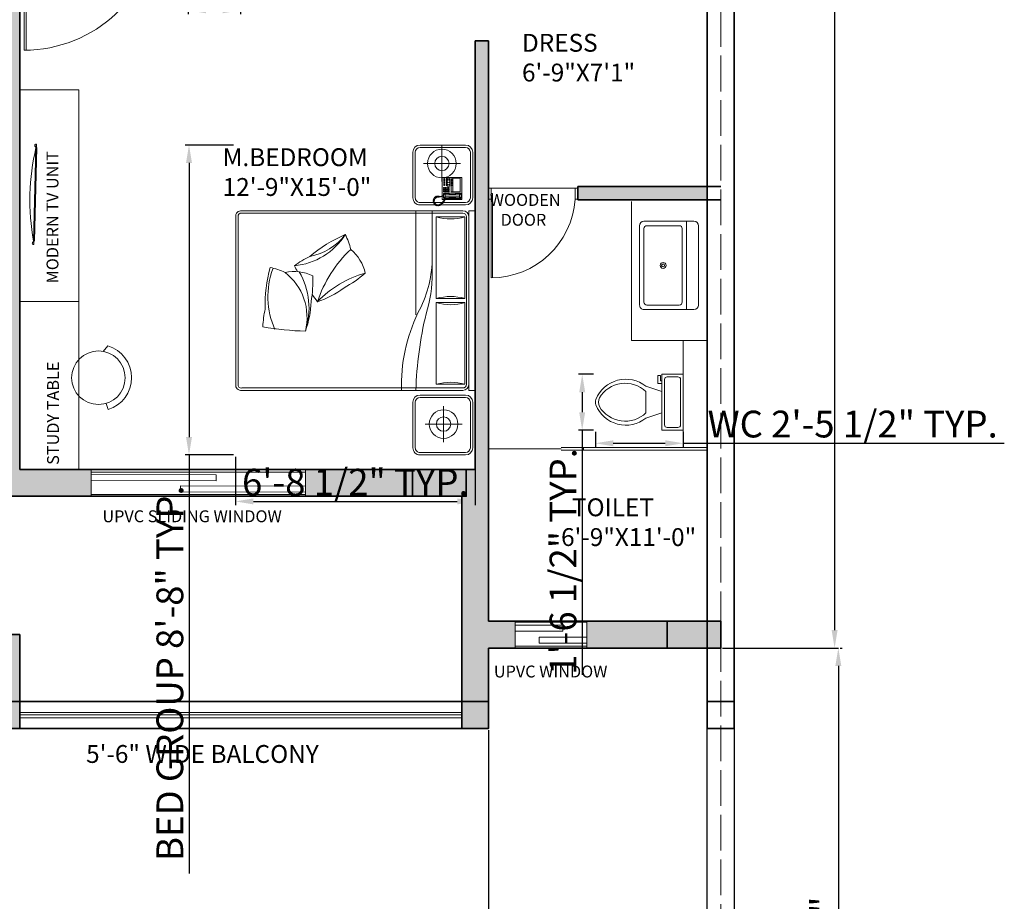
# Model space of a CAD drawing. Units: millimetres. Extents: x 595116 to 630915, y 909473 to 920225.
# Tile 131 of 134: x 630585 to 630915, y 919276 to 919572. Entities that reach past the tile are written whole.
import ezdxf

# ---------------------------------------------------------------- set-up
doc = ezdxf.new("R2010")
doc.units = ezdxf.units.MM
doc.linetypes.add('ACAD_ISO02W100', pattern=[15, 12, -3])
for name, color, linetype, lineweight in [('A-AREA-IDEN', 7, 'Continuous', 20), ('A-EQPM', 8, 'Continuous', 13), ('A-FLOR-BALC', 152, 'Continuous', 18), ('A-FLOR-FIXT', 9, 'Continuous', 18), ('A-FURN', 32, 'Continuous', 18), ('A-WALL', 1, 'Continuous', 35), ('A-WALL-PATT', 8, 'Continuous', 13), ('C-PROP', 7, 'Continuous', 25), ('C-PROP-REF', 240, 'ACAD_ISO02W100', 13), ('Column', 6, 'Continuous', 35), ('Dimension', 3, 'Continuous', 18), ('Doors', 31, 'Continuous', 20), ('Text', 7, 'Continuous', 18), ('Windows', 33, 'Continuous', 18)]:
    doc.layers.add(name, color=color, linetype=linetype, lineweight=lineweight)
doc.styles.get("Standard").update_dxf_attribs({"font": 'arial.ttf'})
doc.dimstyles.new('ISO-25', dxfattribs={"dimtxt": 9, "dimasz": 6, "dimexe": 1.25, "dimexo": 0.625, "dimtad": 1, "dimlunit": 4, "dimtxsty": 'Standard', "dimcen": 2.5, "dimadec": 0, "dimazin": 0, "dimtfac": 1, "dimtmove": 0, "dimatfit": 3, "dimfxl": 1, "dimarcsym": 0})

# ---------------------------------------------------------------- blocks, each defined once
blk = doc.blocks.new('KWD')
for points in [[(629753.63, 919957.93), (629752.54, 919957.93), (629752.54, 919953.43), (629753.63, 919953.43)], [(629787.45, 919957.93), (629787.45, 919953.43), (629788.54, 919953.43), (629788.54, 919957.93)]]:
    blk.add_lwpolyline(points, close=True)
blk.add_lwpolyline([(629753.63, 919921.79), (629753.63, 919955.68), (629754.13, 919955.68), (629754.13, 919921.8)])
blk.add_arc((629753.64, 919955.68), 33.88, 269.99, 356.196)
blk = doc.blocks.new('DS')
blk.add_lwpolyline([(630069.78, 919993.92), (630069.78, 919965.68), (630069.37, 919965.68), (630069.37, 919993.91)])
for points in [[(630041.6, 919963.81), (630041.6, 919967.56), (630040.69, 919967.56), (630040.69, 919963.81)], [(630069.78, 919963.81), (630070.69, 919963.81), (630070.69, 919967.56), (630069.78, 919967.56)]]:
    blk.add_lwpolyline(points, close=True)
blk.add_arc((630069.78, 919965.69), 28.24, 89.99, 176.196)
blk = doc.blocks.new('Toilet - top')
for p, q in [((9.5, -6), (9.5, -2)), ((-10, -8.5), (-8, -8.5)), ((-10, -9.5), (-10, -8.5)), ((-7, -9.5), (-10, -9.5)), ((-8, -8.5), (-8, -8)), ((-7, -8), (-7, -9.5)), ((-4, -8), (-6, -14)), ((4, -8), (6, -14)), ((4, -14), (-4, -14))]:
    blk.add_line(p, q)
blk.add_lwpolyline([(10.5, -8), (10.5, 0), (-10.5, 0), (-10.5, -8)], close=True)
for points in [[(-9.5, -2), (-9.5, -6)], [(8.5, -1), (-8.5, -1)], [(-8.5, -7), (8.5, -7)]]:
    blk.add_lwpolyline(points)
for centre, radius, start, end in [((-8.62, -1.88), 0.884, 81.8699, 188.1301), ((8.62, -1.88), 0.884, 351.8699, 98.1301), ((-8.62, -6.12), 0.884, 171.8699, 278.1301), ((8.62, -6.12), 0.884, 261.8699, 8.1301), ((3.52, -21.58), 12.17, 141.4691, 247.9714), ((4.2, -21.82), 11.33, 136.3677, 238.9468), ((-3.52, -21.58), 12.17, 292.0284, 38.5307), ((-4.2, -21.82), 11.33, 301.053, 43.6321), ((0, -27.88), 4, 245.7318, 294.2682), ((0, -29), 4, 254.8605, 285.1395)]:
    blk.add_arc(centre, radius, start, end)
blk = doc.blocks.new('Sink-single - 30 in top')
blk.add_line((-15, -3.999996), (15, -3.999996))
for points in [[(-13.5, 0), (13.5, 0)], [(-15, -18.499996), (-15, -1.5)], [(15, -1.5), (15, -18.499996)], [(-13.5, -17.499996), (-13.5, -6.499996)], [(-12.5, -5.499996), (12.5, -5.499996)], [(13.5, -6.499996), (13.5, -17.499996)], [(13.5, -19.999996), (-13.5, -19.999996)], [(12.5, -18.499996), (-12.5, -18.499996)]]:
    blk.add_lwpolyline(points)
for radius in [1, 0.5]:
    blk.add_circle((0, -11.999996), radius)
for centre, radius, start, end in [((-13.5, -1.5), 1.5, 90, 180), ((13.5, -1.5), 1.5, 0, 90), ((-12.5, -6.499996), 1, 90, 180), ((12.5, -6.499996), 1, 0, 90), ((-13.5, -18.499996), 1.5, 180, 270), ((-12.5, -17.499996), 1, 180, 270), ((12.5, -17.499996), 1, 270, 0), ((13.5, -18.499996), 1.5, 270, 0)]:
    blk.add_arc(centre, radius, start, end)
blk = doc.blocks.new('A$C356F0359')
for p, q in [((0.4398, 1.9801), (0.0598, 1.9801)), ((0.5489, 2), (2.0492, 2)), ((0.5489, 1.9489), (0.5489, 2)), ((2.0492, 1.9489), (2.0492, 2)), ((2.5283, 1.9801), (2.1483, 1.9801)), ((-0.0002, 1.9201), (-0.0002, 1.5401)), ((0.0198, 1.9201), (0.0198, 1.5401)), ((0.4398, 1.9601), (0.0598, 1.9601)), ((0.4798, 1.5401), (0.4798, 1.9201)), ((0.4998, 1.5401), (0.4998, 1.9201)), ((2.0492, 1.9489), (0.5489, 1.9489)), ((0.5489, 1.8977), (0.5489, 0.0512)), ((0.5689, 1.8977), (0.5689, 0.0512)), ((1.998, 1.9289), (0.6001, 1.9289)), ((2.0292, 0.0512), (2.0292, 1.8977)), ((2.0492, 0.0512), (2.0492, 1.8977)), ((2.0883, 1.9201), (2.0883, 1.5401)), ((2.1083, 1.9201), (2.1083, 1.5401)), ((2.5283, 1.9601), (2.1483, 1.9601)), ((2.5683, 1.5401), (2.5683, 1.9201)), ((2.5883, 1.5401), (2.5883, 1.9201)), ((0.1539, 1.5681), (0.1539, 1.8777)), ((0.2725, 1.8879), (0.2702, 1.8856)), ((0.2702, 1.8856), (0.2702, 1.7279)), ((0.2725, 1.8879), (0.4531, 1.8879)), ((0.3913, 1.8753), (0.277, 1.8753)), ((0.277, 1.8753), (0.277, 1.8147)), ((0.277, 1.8147), (0.3913, 1.8147)), ((0.3913, 1.8125), (0.2816, 1.8125)), ((0.2816, 1.8125), (0.2816, 1.801)), ((0.2907, 1.8125), (0.2907, 1.801)), ((0.2999, 1.8125), (0.2999, 1.801)), ((0.309, 1.8125), (0.309, 1.801)), ((0.3182, 1.8125), (0.3182, 1.801)), ((0.3273, 1.8125), (0.3273, 1.801)), ((0.3365, 1.8125), (0.3365, 1.801)), ((0.3913, 1.8147), (0.3913, 1.8753)), ((0.3913, 1.801), (0.3913, 1.8125)), ((0.4016, 1.8787), (0.4062, 1.8845)), ((0.4016, 1.7404), (0.4016, 1.8787)), ((0.4062, 1.881), (0.405, 1.8765)), ((0.405, 1.8765), (0.4153, 1.8662)), ((0.405, 1.8765), (0.405, 1.8456)), ((0.405, 1.8456), (0.4073, 1.8399)), ((0.4062, 1.8845), (0.4405, 1.8845)), ((0.4108, 1.8833), (0.4062, 1.881)), ((0.4073, 1.8399), (0.4108, 1.8342)), ((0.4108, 1.8833), (0.4382, 1.8833)), ((0.4165, 1.8685), (0.4108, 1.8833)), ((0.4108, 1.8342), (0.4119, 1.8262)), ((0.4119, 1.8262), (0.4119, 1.8147)), ((0.4119, 1.793), (0.4119, 1.8147)), ((0.4153, 1.8662), (0.4165, 1.8685)), ((0.4153, 1.8147), (0.4153, 1.8662)), ((0.4153, 1.8147), (0.4153, 1.753)), ((0.4325, 1.8685), (0.4165, 1.8685)), ((0.4325, 1.8685), (0.4382, 1.8833)), ((0.4336, 1.8662), (0.4325, 1.8685)), ((0.4439, 1.8765), (0.4336, 1.8662)), ((0.4336, 1.8147), (0.4336, 1.8662)), ((0.4336, 1.8147), (0.4336, 1.753)), ((0.4382, 1.8342), (0.4371, 1.8262)), ((0.4371, 1.8262), (0.4371, 1.8147)), ((0.4371, 1.793), (0.4371, 1.8147)), ((0.4382, 1.8833), (0.4428, 1.881)), ((0.4416, 1.8399), (0.4382, 1.8342)), ((0.4405, 1.8845), (0.4462, 1.8787)), ((0.4439, 1.8456), (0.4416, 1.8399)), ((0.4428, 1.881), (0.4439, 1.8765)), ((0.4439, 1.8765), (0.4439, 1.8456)), ((0.4462, 1.8787), (0.4462, 1.7416)), ((0.4531, 1.8879), (0.4553, 1.8856)), ((0.4553, 1.8856), (0.4553, 1.7279)), ((2.3306, 1.5822), (2.3306, 1.8917)), ((0.2702, 1.7279), (0.2725, 1.7256)), ((0.277, 1.7885), (0.277, 1.7679)), ((0.3445, 1.7885), (0.277, 1.7885)), ((0.277, 1.7679), (0.3445, 1.7679)), ((0.2782, 1.7622), (0.2782, 1.7576)), ((0.2896, 1.7622), (0.2782, 1.7622)), ((0.2782, 1.7576), (0.2896, 1.7576)), ((0.2782, 1.745), (0.2896, 1.745)), ((0.2782, 1.7382), (0.2782, 1.745)), ((0.2896, 1.7382), (0.2782, 1.7382)), ((0.2816, 1.801), (0.3913, 1.801)), ((0.2885, 1.7862), (0.2885, 1.7827)), ((0.2919, 1.7862), (0.2885, 1.7862)), ((0.2885, 1.7827), (0.2919, 1.7827)), ((0.2919, 1.7736), (0.2885, 1.7736)), ((0.2885, 1.7736), (0.2885, 1.7702)), ((0.2885, 1.7702), (0.2919, 1.7702)), ((0.2896, 1.7576), (0.2896, 1.7622)), ((0.2896, 1.745), (0.2896, 1.7382)), ((0.2919, 1.7827), (0.2919, 1.7862)), ((0.2919, 1.7702), (0.2919, 1.7736)), ((0.2942, 1.7622), (0.2942, 1.7576)), ((0.3056, 1.7622), (0.2942, 1.7622)), ((0.2942, 1.7576), (0.3056, 1.7576)), ((0.2942, 1.745), (0.3056, 1.745)), ((0.2942, 1.7382), (0.2942, 1.745)), ((0.3056, 1.7382), (0.2942, 1.7382)), ((0.3056, 1.7576), (0.3056, 1.7622)), ((0.3056, 1.745), (0.3056, 1.7382)), ((0.3125, 1.7862), (0.309, 1.7862)), ((0.309, 1.7862), (0.309, 1.7827)), ((0.309, 1.7827), (0.3125, 1.7827)), ((0.3125, 1.7736), (0.309, 1.7736)), ((0.309, 1.7736), (0.309, 1.7702)), ((0.309, 1.7702), (0.3125, 1.7702)), ((0.3102, 1.7622), (0.3102, 1.7576)), ((0.3216, 1.7622), (0.3102, 1.7622)), ((0.3102, 1.7576), (0.3216, 1.7576)), ((0.3102, 1.745), (0.3216, 1.745)), ((0.3102, 1.7382), (0.3102, 1.745)), ((0.3216, 1.7382), (0.3102, 1.7382)), ((0.3125, 1.7827), (0.3125, 1.7862)), ((0.3125, 1.7702), (0.3125, 1.7736)), ((0.3216, 1.7576), (0.3216, 1.7622)), ((0.3216, 1.745), (0.3216, 1.7382)), ((0.3376, 1.7622), (0.3262, 1.7622)), ((0.3262, 1.7622), (0.3262, 1.7576)), ((0.3262, 1.7576), (0.3376, 1.7576)), ((0.3262, 1.7382), (0.3262, 1.745)), ((0.3262, 1.745), (0.3376, 1.745)), ((0.3376, 1.7382), (0.3262, 1.7382)), ((0.333, 1.7862), (0.3296, 1.7862)), ((0.3296, 1.7862), (0.3296, 1.7827)), ((0.3296, 1.7827), (0.333, 1.7827)), ((0.333, 1.7736), (0.3296, 1.7736)), ((0.3296, 1.7736), (0.3296, 1.7702)), ((0.3296, 1.7702), (0.333, 1.7702)), ((0.333, 1.7827), (0.333, 1.7862)), ((0.333, 1.7702), (0.333, 1.7736)), ((0.3376, 1.7576), (0.3376, 1.7622)), ((0.3376, 1.745), (0.3376, 1.7382)), ((0.3445, 1.7679), (0.3445, 1.7885)), ((0.3548, 1.7759), (0.3548, 1.7827)), ((0.3548, 1.7827), (0.3639, 1.7827)), ((0.3639, 1.7759), (0.3548, 1.7759)), ((0.3548, 1.7633), (0.3548, 1.7702)), ((0.3548, 1.7702), (0.3639, 1.7702)), ((0.3639, 1.7633), (0.3548, 1.7633)), ((0.3548, 1.7564), (0.3639, 1.7564)), ((0.3548, 1.7496), (0.3548, 1.7564)), ((0.3639, 1.7496), (0.3548, 1.7496)), ((0.3548, 1.737), (0.3548, 1.7439)), ((0.3548, 1.7439), (0.3639, 1.7439)), ((0.3639, 1.737), (0.3548, 1.737)), ((0.3639, 1.7827), (0.3639, 1.7759)), ((0.3639, 1.7702), (0.3639, 1.7633)), ((0.3639, 1.7564), (0.3639, 1.7496)), ((0.3639, 1.7439), (0.3639, 1.737)), ((0.3685, 1.7827), (0.3776, 1.7827)), ((0.3685, 1.7759), (0.3685, 1.7827)), ((0.3776, 1.7759), (0.3685, 1.7759)), ((0.3685, 1.7633), (0.3685, 1.7702)), ((0.3685, 1.7702), (0.3776, 1.7702)), ((0.3776, 1.7633), (0.3685, 1.7633)), ((0.3685, 1.7564), (0.3776, 1.7564)), ((0.3685, 1.7496), (0.3685, 1.7564)), ((0.3776, 1.7496), (0.3685, 1.7496)), ((0.3685, 1.737), (0.3685, 1.7439)), ((0.3685, 1.7439), (0.3776, 1.7439)), ((0.3776, 1.737), (0.3685, 1.737)), ((0.3776, 1.7827), (0.3776, 1.7759)), ((0.3776, 1.7702), (0.3776, 1.7633)), ((0.3776, 1.7564), (0.3776, 1.7496)), ((0.3776, 1.7439), (0.3776, 1.737)), ((0.3822, 1.7759), (0.3822, 1.7827)), ((0.3822, 1.7827), (0.3913, 1.7827)), ((0.3913, 1.7759), (0.3822, 1.7759)), ((0.3822, 1.7633), (0.3822, 1.7702)), ((0.3822, 1.7702), (0.3913, 1.7702)), ((0.3913, 1.7633), (0.3822, 1.7633)), ((0.3822, 1.7576), (0.3913, 1.7576)), ((0.3822, 1.7507), (0.3822, 1.7576)), ((0.3913, 1.7507), (0.3822, 1.7507)), ((0.3822, 1.7439), (0.3913, 1.7439)), ((0.3822, 1.737), (0.3822, 1.7439)), ((0.3913, 1.737), (0.3822, 1.737)), ((0.3913, 1.7827), (0.3913, 1.7759)), ((0.3913, 1.7702), (0.3913, 1.7633)), ((0.3913, 1.7576), (0.3913, 1.7507)), ((0.3913, 1.7439), (0.3913, 1.737)), ((0.4073, 1.7347), (0.4016, 1.7404)), ((0.405, 1.7736), (0.4073, 1.7793)), ((0.405, 1.7427), (0.405, 1.7736)), ((0.405, 1.7427), (0.4153, 1.753)), ((0.4062, 1.7382), (0.405, 1.7427)), ((0.4108, 1.7359), (0.4062, 1.7382)), ((0.4073, 1.7793), (0.4108, 1.785)), ((0.4234, 1.7347), (0.4073, 1.7347)), ((0.4108, 1.785), (0.4119, 1.793)), ((0.4165, 1.7507), (0.4108, 1.7359)), ((0.4108, 1.7359), (0.4234, 1.7359)), ((0.4153, 1.753), (0.4165, 1.7507)), ((0.4325, 1.7507), (0.4165, 1.7507)), ((0.4233, 1.7393), (0.4235, 1.7294)), ((0.4268, 1.7393), (0.4233, 1.7393)), ((0.4235, 1.7294), (0.4263, 1.7179)), ((0.4274, 1.7301), (0.4268, 1.7393)), ((0.427, 1.7359), (0.4382, 1.7359)), ((0.4405, 1.7347), (0.4271, 1.7347)), ((0.429, 1.7227), (0.4274, 1.7301)), ((0.4336, 1.753), (0.4325, 1.7507)), ((0.4325, 1.7507), (0.4382, 1.7359)), ((0.4439, 1.7427), (0.4336, 1.753)), ((0.4382, 1.785), (0.4371, 1.793)), ((0.4416, 1.7793), (0.4382, 1.785)), ((0.4382, 1.7359), (0.4428, 1.7382)), ((0.4462, 1.7416), (0.4405, 1.7347)), ((0.4439, 1.7736), (0.4416, 1.7793)), ((0.4428, 1.7382), (0.4439, 1.7427)), ((0.4439, 1.7427), (0.4439, 1.7736)), ((0.4553, 1.7279), (0.4531, 1.7256)), ((0.4622, 1.7459), (0.4553, 1.7484)), ((0.4553, 1.7439), (0.4604, 1.7425)), ((0.4604, 1.7425), (0.465, 1.7388)), ((0.4654, 1.7427), (0.4622, 1.7459)), ((0.465, 1.7388), (0.4662, 1.7372)), ((0.4678, 1.7405), (0.4654, 1.7427)), ((0.4662, 1.7372), (0.4686, 1.7374)), ((0.4686, 1.7374), (0.4662, 1.735)), ((0.4662, 1.735), (0.4755, 1.7268)), ((0.4721, 1.7421), (0.4678, 1.7405)), ((0.4741, 1.7401), (0.4721, 1.7421)), ((0.4725, 1.7366), (0.4741, 1.7401)), ((0.4753, 1.7388), (0.4725, 1.7366)), ((0.4783, 1.7356), (0.4753, 1.7388)), ((0.4759, 1.729), (0.4783, 1.7356)), ((0.4821, 1.7322), (0.4759, 1.729)), ((0.4874, 1.7272), (0.4821, 1.7322)), ((2.4819, 1.7366), (2.1818, 1.7366)), ((0.3052, 1.7226), (0.0051, 1.7226)), ((0.4244, 1.7256), (0.2725, 1.7256)), ((0.4263, 1.7179), (0.429, 1.707)), ((0.427, 1.697), (0.4265, 1.6915)), ((0.4265, 1.6915), (0.4332, 1.6903)), ((0.4332, 1.6903), (0.4267, 1.6864)), ((0.4267, 1.6864), (0.4272, 1.6801)), ((0.4295, 1.6996), (0.427, 1.697)), ((0.4272, 1.6801), (0.4346, 1.6794)), ((0.4346, 1.6794), (0.4281, 1.6744)), ((0.4281, 1.6744), (0.4311, 1.669)), ((0.4531, 1.7256), (0.4284, 1.7256)), ((0.429, 1.707), (0.4288, 1.701)), ((0.4288, 1.701), (0.4295, 1.6996)), ((0.4318, 1.7119), (0.429, 1.7227)), ((0.4311, 1.669), (0.4381, 1.6704)), ((0.4325, 1.7063), (0.4318, 1.7119)), ((0.4323, 1.7003), (0.4325, 1.7063)), ((0.4364, 1.6973), (0.4323, 1.7003)), ((0.4381, 1.6704), (0.4348, 1.6639)), ((0.4348, 1.6639), (0.4383, 1.6598)), ((0.4355, 1.6919), (0.4364, 1.6973)), ((0.4367, 1.6774), (0.4355, 1.6919)), ((0.4455, 1.6663), (0.4367, 1.6774)), ((0.4383, 1.6598), (0.4436, 1.6637)), ((0.4436, 1.6637), (0.4427, 1.6575)), ((0.4427, 1.6575), (0.4471, 1.6547)), ((0.4577, 1.6598), (0.4455, 1.6663)), ((0.4471, 1.6547), (0.4526, 1.6593)), ((0.4526, 1.6593), (0.4519, 1.6517)), ((0.4519, 1.6517), (0.4568, 1.6503)), ((0.4568, 1.6503), (0.4598, 1.6565)), ((0.4716, 1.6586), (0.4577, 1.6598)), ((0.4598, 1.6565), (0.4626, 1.6503)), ((0.4626, 1.6503), (0.4665, 1.6498)), ((0.4665, 1.6498), (0.4681, 1.6565)), ((0.4681, 1.6565), (0.4707, 1.6491)), ((0.4707, 1.6491), (0.4751, 1.6503)), ((0.485, 1.6644), (0.4716, 1.6586)), ((0.4751, 1.6503), (0.4753, 1.6565)), ((0.4753, 1.6565), (0.4806, 1.6519)), ((0.4755, 1.7268), (0.4906, 1.7139)), ((0.4806, 1.6519), (0.4843, 1.6538)), ((0.4843, 1.6538), (0.4836, 1.6607)), ((0.4836, 1.6607), (0.4885, 1.6547)), ((0.4952, 1.6744), (0.485, 1.6644)), ((0.4862, 1.7199), (0.4874, 1.7272)), ((0.4914, 1.7231), (0.4862, 1.7199)), ((0.4885, 1.6547), (0.4922, 1.6579)), ((0.4922, 1.6579), (0.4894, 1.6642)), ((0.4894, 1.6642), (0.4959, 1.6614)), ((0.4908, 1.7135), (0.4984, 1.6917)), ((0.4958, 1.7185), (0.4914, 1.7231)), ((0.494, 1.7135), (0.4958, 1.7185)), ((0.501, 1.7142), (0.494, 1.7135)), ((0.4984, 1.6917), (0.4952, 1.6744)), ((0.4957, 1.6704), (0.5024, 1.6683)), ((0.4989, 1.6642), (0.4957, 1.6704)), ((0.4959, 1.6614), (0.4989, 1.6642)), ((0.4964, 1.7047), (0.5031, 1.7072)), ((0.5038, 1.7049), (0.4964, 1.7047)), ((0.5042, 1.673), (0.4987, 1.6792)), ((0.4987, 1.6792), (0.5058, 1.679)), ((0.5005, 1.695), (0.5054, 1.6996)), ((0.5068, 1.695), (0.5005, 1.695)), ((0.5008, 1.6871), (0.5079, 1.6892)), ((0.5068, 1.6836), (0.5008, 1.6871)), ((0.5031, 1.7072), (0.501, 1.7142)), ((0.5024, 1.6683), (0.5042, 1.673)), ((0.5054, 1.6996), (0.5038, 1.7049)), ((0.5058, 1.679), (0.5068, 1.6836)), ((0.5079, 1.6892), (0.5068, 1.695)), ((0.0598, 1.5001), (0.4398, 1.5001)), ((2.1483, 1.5001), (2.5283, 1.5001)), ((0.0598, 1.4801), (0.4398, 1.4801)), ((2.1483, 1.4801), (2.5283, 1.4801)), ((0.6001, 0.02), (1.998, 0.02)), ((0.6001, 0), (1.998, 0))]:
    blk.add_line(p, q)
at = {"linetype": 'ByBlock'}
for p, q in [((0.6001, 1.9147), (1.282, 1.9147)), ((0.6001, 1.6759), (0.6001, 1.9147)), ((1.282, 1.9147), (1.282, 1.6759)), ((1.3161, 1.9147), (1.998, 1.9147)), ((1.3161, 1.6759), (1.3161, 1.9147)), ((1.998, 1.9147), (1.998, 1.6759)), ((1.282, 1.6759), (0.6001, 1.6759)), ((1.998, 1.6759), (1.3161, 1.6759)), ((1.0687, 1.6418), (0.5489, 1.6418)), ((1.4185, 1.5053), (0.5489, 1.5053))]:
    blk.add_line(p, q, dxfattribs=at)
for centre in [(0.1539, 1.7226), (2.3306, 1.7366)]:
    blk.add_circle(centre, 0.12, dxfattribs=at)
for centre in [(0.1539, 1.7226), (2.3306, 1.7366)]:
    blk.add_circle(centre, 0.06)
for centre, radius, start, end in [((0.0598, 1.9201), 0.06, 90, 180), ((0.4398, 1.9201), 0.06, 0, 90), ((2.1483, 1.9201), 0.06, 90, 180), ((2.5283, 1.9201), 0.06, 0, 90), ((0.0598, 1.9201), 0.04, 90, 180), ((0.4398, 1.9201), 0.04, 0, 90), ((0.6001, 1.8977), 0.0512, 90, 180), ((0.6001, 1.8977), 0.0312, 90, 180), ((1.998, 1.8977), 0.0512, 0, 90), ((1.998, 1.8977), 0.0312, 0, 90), ((2.1483, 1.9201), 0.04, 90, 180), ((2.5283, 1.9201), 0.04, 0, 90), ((0.0598, 1.5401), 0.06, 180, 270), ((0.0598, 1.5401), 0.04, 180, 270), ((0.4398, 1.5401), 0.04, 270, 0), ((0.4398, 1.5401), 0.06, 270, 0), ((2.1483, 1.5401), 0.06, 180, 270), ((2.1483, 1.5401), 0.04, 180, 270), ((2.5283, 1.5401), 0.06, 270, 0), ((2.5283, 1.5401), 0.04, 270, 0), ((1.1471, 0.7332), 0.3575, 102.47819, 140.46254), ((1.9086, 1.3124), 0.8697, 195.33601, 226.41927), ((0.3249, 0.4335), 0.9879, 28.49711, 41.05657), ((0.9965, 0.4273), 0.548, 103.20343, 117.03623), ((0.4451, 0.4375), 0.5655, 5.33912, 57.68949), ((0.4517, 0.5274), 0.4879, 10.69865, 52.68638), ((1.8195, 1.3719), 1.1652, 203.06416, 220.32086), ((1.6529, 1.7059), 1.0798, 223.63057, 251.4288), ((0.5617, 0.4344), 0.7874, 18.35266, 36.68512), ((-0.021, 2.4319), 2.1977, 305.29657, 307.24182), ((1.5949, 0.9312), 0.734, 205.25901, 216.93514), ((1.4135, 0.487), 0.3575, 154.0418, 192.02615), ((1.3641, 0.0041), 0.6085, 71.81005, 120.13512), ((1.44, 0.1186), 0.4774, 76.18494, 142.00166), ((1.1372, -0.3434), 0.9879, 80.06073, 92.62018), ((1.2836, -0.1573), 0.7874, 69.91627, 88.24873), ((-0.6432, 0.628), 2.1977, 349.48843, 358.80544), ((-0.021, 2.4319), 2.1977, 297.92482, 299.3793), ((1.5595, 0.1789), 0.548, 154.76704, 168.59984), ((1.3312, 1.4107), 1.1652, 254.62778, 271.88448), ((1.2647, 0.9578), 0.6885, 250.29361, 293.6414), ((1.5368, 0.9609), 0.734, 256.82263, 268.49876), ((0.5943, 0.0454), 0.0458, 172.75992, 277.24008), ((0.5943, 0.0454), 0.0258, 172.75992, 277.24008), ((2.0038, 0.0454), 0.0458, 262.75992, 7.24008), ((2.0038, 0.0454), 0.0258, 262.75992, 7.24008)]:
    blk.add_arc(centre, radius, start, end)
for centre, radius, start, end in [((0.1906, 1.7953), 0.4265, 343.73979, 16.26021), ((1.6914, 1.7953), 0.4265, 163.73979, 196.26021), ((0.9067, 1.7953), 0.4265, 343.73979, 16.26021), ((2.4075, 1.7953), 0.4265, 163.73979, 196.26021), ((0.9303, 0.657), 0.9853, 61.43285, 88.12613), ((1.0826, 0.5712), 1.0706, 72.19663, 90.74184), ((2.1368, 4.5996), 3.0955, 256.42012, 268.37887), ((2.0056, 2.7745), 1.3903, 244.24266, 271.79845)]:
    blk.add_arc(centre, radius, start, end, dxfattribs=at)
blk = doc.blocks.new('*D131')
at = {"layer": 'Defpoints', "color": 0, "transparency": 16777216}
for p in [(630820.1, 919957.93), (630820.1, 919360.93), (630858.37, 919360.93)]:
    blk.add_point(p, dxfattribs=at)
at = {"layer": 'Dimension', "color": 0, "lineweight": -2, "transparency": 16777216}
for p, q in [((630820.72, 919957.93), (630859.62, 919957.93)), ((630858.37, 919951.93), (630858.37, 919366.93)), ((630820.72, 919360.93), (630859.62, 919360.93))]:
    blk.add_line(p, q, dxfattribs=at)
at = {"layer": 'Dimension', "color": 0, "transparency": 16777216}
for points in [[(630857.37, 919951.93), (630859.37, 919951.93), (630858.37, 919957.93)], [(630857.37, 919366.93), (630859.37, 919366.93), (630858.37, 919360.93)]]:
    blk.add_solid(points, dxfattribs=at)
at = {"layer": 'Dimension', "color": 0, "transparency": 16777216, "insert": (630853.15, 919659.43), "char_height": 9, "attachment_point": 5, "rotation": 90}
blk.add_mtext('49\'-9"', dxfattribs=at)
blk = doc.blocks.new('*D132')
at = {"layer": 'Defpoints', "color": 0, "transparency": 16777216}
for p in [(630859.62, 919360.93), (630859.62, 919146.43), (630859.62, 919146.43)]:
    blk.add_point(p, dxfattribs=at)
at = {"layer": 'Dimension', "color": 0, "lineweight": -2, "transparency": 16777216}
for p, q in [((630860.25, 919360.93), (630860.87, 919360.93)), ((630859.62, 919354.93), (630859.62, 919152.43)), ((630860.25, 919146.43), (630860.87, 919146.43))]:
    blk.add_line(p, q, dxfattribs=at)
at = {"layer": 'Dimension', "color": 0, "transparency": 16777216}
for points in [[(630858.62, 919354.93), (630860.62, 919354.93), (630859.62, 919360.93)], [(630858.62, 919152.43), (630860.62, 919152.43), (630859.62, 919146.43)]]:
    blk.add_solid(points, dxfattribs=at)
at = {"layer": 'Dimension', "color": 0, "transparency": 16777216, "insert": (630848.38, 919253.68), "char_height": 9, "attachment_point": 5, "rotation": 90}
blk.add_mtext('17\'-10{\\H1x;\\S1/2;}"', dxfattribs=at)
blk = doc.blocks.new('TV-SCREEN')
for p, q in [((2.14, 32.58), (2.14, 33.76)), ((2.19, 32.58), (2.19, 33.76)), ((2.04, 32.58), (1.21, 1.19)), ((2.14, 32.58), (1.31, 1.19)), ((2.24, 32.58), (1.41, 1.19)), ((2.34, 32.57), (1.51, 1.18)), ((1.31, 1.19), (1.31, 0.01)), ((1.36, 1.19), (1.36, 0.01))]:
    blk.add_line(p, q)
for centre, radius, start, end in [((2.09, 33.31), 0.462, 77.1755, 282.8245), ((76.63, 14.9), 76.65, 166.662, 190.3006), ((1.26, 0.46), 0.462, 77.1755, 282.8245)]:
    blk.add_arc(centre, radius, start, end)
blk = doc.blocks.new('CHAIR-ROUND-2')
for p, q in [((12.11, 21.41), (10.53, 19.55)), ((12.22, 0), (11.59, 2.08))]:
    blk.add_line(p, q)
blk.add_circle((8.99, 10.69), 8.99)
blk.add_arc((8.99, 10.69), 11.16, 286.7943, 73.7898)
blk = doc.blocks.new('COLUMN-SQUARE-9IN')
h = blk.add_hatch(color=256)
h.dxf.hatch_style = 1
h.paths.add_polyline_path([(9, 9), (0, 9), (0, 0), (9, 0)])
blk.add_lwpolyline([(0, 9), (9, 9), (9, 0), (0, 0)], close=True)
blk = doc.blocks.new('COLUMN-RECT-18X9')
h = blk.add_hatch(color=256)
h.dxf.hatch_style = 1
h.paths.add_polyline_path([(18, 9), (0, 9), (0, 0), (18, 0)])
blk.add_lwpolyline([(0, 9), (18, 9), (18, 0), (0, 0)], close=True)
blk = doc.blocks.new('*D168')
at = {"layer": 'Defpoints', "color": 0, "transparency": 16777216}
for p in [(630657.1, 919529.88), (630641.48, 919425.79), (630657.1, 919425.79)]:
    blk.add_point(p, dxfattribs=at)
at = {"layer": 'Dimension', "color": 0, "lineweight": -2, "transparency": 16777216}
for p, q in [((630656.47, 919529.88), (630640.23, 919529.88)), ((630641.48, 919523.88), (630641.48, 919431.79)), ((630656.47, 919425.79), (630640.23, 919425.79)), ((630641.48, 919425.79), (630641.48, 919285.14))]:
    blk.add_line(p, q, dxfattribs=at)
at = {"layer": 'Dimension', "color": 0, "transparency": 16777216}
for points in [[(630640.48, 919523.88), (630642.48, 919523.88), (630641.48, 919529.88)], [(630640.48, 919431.79), (630642.48, 919431.79), (630641.48, 919425.79)]]:
    blk.add_solid(points, dxfattribs=at)
at = {"layer": 'Dimension', "color": 0, "transparency": 16777216, "insert": (630636.2, 919352.46), "char_height": 9, "attachment_point": 5, "rotation": 90}
blk.add_mtext('BED GROUP 8\'-8" TYP.', dxfattribs=at)
blk = doc.blocks.new('*D169')
at = {"layer": 'Defpoints', "color": 0, "transparency": 16777216}
for p in [(630657.1, 919425.79), (630737.6, 919425.79), (630737.6, 919410.18)]:
    blk.add_point(p, dxfattribs=at)
at = {"layer": 'Dimension', "color": 0, "lineweight": -2, "transparency": 16777216}
for p, q in [((630657.1, 919425.17), (630657.1, 919408.93)), ((630737.6, 919425.17), (630737.6, 919408.93)), ((630663.1, 919410.18), (630731.6, 919410.18))]:
    blk.add_line(p, q, dxfattribs=at)
at = {"layer": 'Dimension', "color": 0, "transparency": 16777216}
for points in [[(630663.1, 919411.18), (630663.1, 919409.18), (630657.1, 919410.18)], [(630731.6, 919411.18), (630731.6, 919409.18), (630737.6, 919410.18)]]:
    blk.add_solid(points, dxfattribs=at)
at = {"layer": 'Dimension', "color": 0, "transparency": 16777216, "insert": (630697.35, 919415.46), "char_height": 9, "attachment_point": 5}
blk.add_mtext('6\'-8 1/2" TYP.', dxfattribs=at)
blk = doc.blocks.new('*D172')
at = {"layer": 'Defpoints', "color": 0, "transparency": 16777216}
for p in [(630777.99, 919434.13), (630807.49, 919434.13), (630807.49, 919429.71)]:
    blk.add_point(p, dxfattribs=at)
at = {"layer": 'Dimension', "color": 0, "lineweight": -2, "transparency": 16777216}
for p, q in [((630777.99, 919433.51), (630777.99, 919428.46)), ((630807.49, 919433.51), (630807.49, 919428.46)), ((630783.99, 919429.71), (630801.49, 919429.71)), ((630807.49, 919429.71), (630915.38, 919429.71))]:
    blk.add_line(p, q, dxfattribs=at)
at = {"layer": 'Dimension', "color": 0, "transparency": 16777216}
for points in [[(630783.99, 919430.71), (630783.99, 919428.71), (630777.99, 919429.71)], [(630801.49, 919430.71), (630801.49, 919428.71), (630807.49, 919429.71)]]:
    blk.add_solid(points, dxfattribs=at)
at = {"layer": 'Dimension', "color": 0, "transparency": 16777216, "insert": (630864.43, 919434.99), "char_height": 9, "attachment_point": 5}
blk.add_mtext('WC 2\'-5 1/2" TYP.', dxfattribs=at)
blk = doc.blocks.new('*D173')
at = {"layer": 'Defpoints', "color": 0, "transparency": 16777216}
for p in [(630777.99, 919452.87), (630773.57, 919434.13), (630777.99, 919434.13)]:
    blk.add_point(p, dxfattribs=at)
at = {"layer": 'Dimension', "color": 0, "lineweight": -2, "transparency": 16777216}
for p, q in [((630777.37, 919452.87), (630772.32, 919452.87)), ((630773.57, 919446.87), (630773.57, 919440.13)), ((630777.37, 919434.13), (630772.32, 919434.13)), ((630773.57, 919434.13), (630773.57, 919351.9))]:
    blk.add_line(p, q, dxfattribs=at)
at = {"layer": 'Dimension', "color": 0, "transparency": 16777216}
for points in [[(630772.57, 919446.87), (630774.57, 919446.87), (630773.57, 919452.87)], [(630772.57, 919440.13), (630774.57, 919440.13), (630773.57, 919434.13)]]:
    blk.add_solid(points, dxfattribs=at)
at = {"layer": 'Dimension', "color": 0, "transparency": 16777216, "insert": (630768.29, 919390.01), "char_height": 9, "attachment_point": 5, "rotation": 90}
blk.add_mtext('1\'-6 1/2" TYP.', dxfattribs=at)
blk = doc.blocks.new('*D207')
at = {"layer": 'Defpoints', "color": 0, "transparency": 16777216}
for p in [(630641.24, 919577.87), (630658.82, 919577.87), (630658.82, 919575.15)]:
    blk.add_point(p, dxfattribs=at)
at = {"layer": 'Dimension', "color": 0, "lineweight": -2, "transparency": 16777216}
for p, q in [((630641.24, 919577.25), (630641.24, 919573.9)), ((630647.24, 919575.15), (630652.82, 919575.15)), ((630658.82, 919577.25), (630658.82, 919573.9)), ((630658.82, 919575.15), (630741.05, 919575.15))]:
    blk.add_line(p, q, dxfattribs=at)
at = {"layer": 'Dimension', "color": 0, "transparency": 16777216}
for points in [[(630647.24, 919576.15), (630647.24, 919574.15), (630641.24, 919575.15)], [(630652.82, 919576.15), (630652.82, 919574.15), (630658.82, 919575.15)]]:
    blk.add_solid(points, dxfattribs=at)
at = {"layer": 'Dimension', "color": 0, "transparency": 16777216, "insert": (630702.94, 919580.43), "char_height": 9, "attachment_point": 5}
blk.add_mtext('1\'-5 1/2" TYP.', dxfattribs=at)
blk = doc.blocks.new('*D218')
at = {"layer": 'Defpoints', "color": 0, "transparency": 16777216}
for p in [(630575.6, 919333.93), (630742.1, 919333.93), (630742.1, 919078.13)]:
    blk.add_point(p, dxfattribs=at)
at = {"layer": 'Dimension', "color": 0, "lineweight": -2, "transparency": 16777216}
for p, q in [((630575.6, 919333.3), (630575.6, 919076.88)), ((630742.1, 919333.3), (630742.1, 919076.88)), ((630581.6, 919078.13), (630736.1, 919078.13))]:
    blk.add_line(p, q, dxfattribs=at)
at = {"layer": 'Dimension', "color": 0, "transparency": 16777216}
for points in [[(630581.6, 919079.13), (630581.6, 919077.13), (630575.6, 919078.13)], [(630736.1, 919079.13), (630736.1, 919077.13), (630742.1, 919078.13)]]:
    blk.add_solid(points, dxfattribs=at)
at = {"layer": 'Dimension', "color": 0, "transparency": 16777216, "insert": (630658.85, 919083.41), "char_height": 9, "attachment_point": 5}
blk.add_mtext('13\'-10 1/2"', dxfattribs=at)

msp = doc.modelspace()

# ---------------------------------------------------------------- hatches: boundary and pattern name
at = {"layer": 'A-WALL-PATT'}
h = msp.add_hatch(color=256, dxfattribs=at)
h.dxf.hatch_style = 1
h.paths.add_polyline_path([(630584.596, 919609.928), (630577.096, 919609.928), (630577.096, 919591.928), (630575.596, 919591.928), (630575.596, 919552.928), (630533.596, 919552.928), (630533.596, 919548.428), (630575.596, 919548.428), (630575.596, 919429.928), (630577.096, 919429.928), (630577.096, 919411.928), (630608.596, 919411.928), (630608.596, 919420.928), (630584.596, 919420.928)])
h = msp.add_hatch(color=256, dxfattribs=at)
h.dxf.hatch_style = 1
h.paths.add_polyline_path([(630742.096, 919564.928), (630737.596, 919564.928), (630737.596, 919420.928), (630734.596, 919420.928), (630734.596, 919411.928), (630733.096, 919411.928), (630733.096, 919342.928), (630742.096, 919342.928), (630742.096, 919360.928), (630751.096, 919360.928), (630751.096, 919369.928), (630742.096, 919369.928)])
h = msp.add_hatch(color=256, dxfattribs=at)
h.dxf.hatch_style = 1
h.paths.add_polyline_path([(630815.596, 919515.928), (630772.096, 919515.928), (630772.096, 919511.428), (630815.596, 919511.428)])
h = msp.add_hatch(color=256, dxfattribs=at)
h.dxf.hatch_style = 1
h.paths.add_polyline_path([(630716.596, 919420.928), (630680.596, 919420.928), (630680.596, 919411.928), (630716.596, 919411.928)])
h = msp.add_hatch(color=256, dxfattribs=at)
h.dxf.hatch_style = 1
h.paths.add_polyline_path([(630802.096, 919369.928), (630775.096, 919369.928), (630775.096, 919360.928), (630802.096, 919360.928)])
h = msp.add_hatch(color=256, dxfattribs=at)
h.dxf.hatch_style = 1
h.paths.add_polyline_path([(630584.596, 919365.428), (630563.266, 919365.428), (630563.266, 919360.928), (630575.596, 919360.928), (630575.596, 919342.928), (630584.596, 919342.928)])

# ---------------------------------------------------------------- linework, layer by layer
at = {"layer": 'A-FLOR-BALC'}
for p, q in [((630733.096, 919339.271), (630584.596, 919339.271)), ((630584.596, 919338.428), (630733.096, 919338.428)), ((630584.596, 919337.435), (630733.096, 919337.435))]:
    msp.add_line(p, q, dxfattribs=at)
at = {"layer": 'A-FLOR-FIXT'}
for p, q in [((630790.096, 919510.928), (630790.096, 919464.269)), ((630790.096, 919464.269), (630815.596, 919464.269)), ((630807.487, 919464.269), (630807.487, 919428.297)), ((630766.465, 919427.855), (630742.096, 919427.855)), ((630815.596, 919428.297), (630766.465, 919428.297)), ((630815.596, 919427.413), (630766.465, 919427.413)), ((630773.965, 919428.297), (630773.965, 919427.413))]:
    msp.add_line(p, q, dxfattribs=at)
at = {"layer": 'A-FURN'}
for p, q in [((630604.483, 919548.428), (630584.596, 919548.428)), ((630604.483, 919548.428), (630604.483, 919420.928)), ((630584.596, 919477.294), (630604.483, 919477.294))]:
    msp.add_line(p, q, dxfattribs=at)
at = {"layer": 'A-WALL'}
for p, q in [((630815.596, 920020.393), (630815.596, 919333.928)), ((630584.596, 919420.928), (630584.596, 919609.928)), ((630737.596, 919420.928), (630737.596, 919564.928)), ((630737.596, 919564.928), (630742.096, 919564.928)), ((630742.096, 919369.928), (630742.096, 919564.928)), ((630772.096, 919515.928), (630820.096, 919515.928)), ((630772.096, 919511.428), (630772.096, 919515.928)), ((630772.096, 919511.428), (630820.096, 919511.428)), ((630584.596, 919420.928), (630737.596, 919420.928)), ((630494.596, 919411.928), (630733.096, 919411.928)), ((630733.096, 919342.928), (630733.096, 919411.928)), ((630742.096, 919369.928), (630820.096, 919369.928)), ((630584.596, 919365.428), (630563.266, 919365.428)), ((630584.596, 919365.428), (630584.596, 919342.928)), ((630742.096, 919333.928), (630742.096, 919360.928)), ((630742.096, 919360.928), (630820.096, 919360.928)), ((630584.596, 919342.928), (630733.096, 919342.928)), ((630815.596, 919342.928), (630824.596, 919342.928)), ((630575.596, 919333.928), (630742.096, 919333.928)), ((630815.596, 919333.928), (630824.596, 919333.928))]:
    msp.add_line(p, q, dxfattribs=at)
msp.add_lwpolyline([(630824.596, 920020.393), (630824.596, 919333.928)], dxfattribs=at)
at = {"layer": 'C-PROP'}
for p, q in [((630815.596, 919155.428), (630815.596, 919333.928)), ((630824.596, 919333.928), (630824.596, 919146.428))]:
    msp.add_line(p, q, dxfattribs=at)
at = {"layer": 'C-PROP-REF'}
msp.add_line((630820.096, 920084.928), (630820.096, 919150.928), dxfattribs=at)
at = {"layer": 'Doors'}
msp.add_line((630743.007, 919515.428), (630771.185, 919515.428), dxfattribs=at)
at = {"layer": 'Windows'}
for p, q in [((630608.596, 919420.928), (630680.596, 919420.928)), ((630608.596, 919420.928), (630608.596, 919411.928)), ((630680.596, 919420.928), (630680.596, 919411.928)), ((630608.598, 919417.165), (630650.596, 919417.079)), ((630608.602, 919419.165), (630650.596, 919419.079)), ((630650.596, 919419.079), (630650.596, 919417.079)), ((630638.596, 919415.357), (630680.594, 919415.271)), ((630638.596, 919415.357), (630638.596, 919413.357)), ((630638.596, 919413.357), (630680.59, 919413.271)), ((630608.596, 919411.928), (630680.596, 919411.928)), ((630751.096, 919369.928), (630775.096, 919369.928)), ((630751.096, 919369.928), (630751.096, 919360.928)), ((630775.096, 919369.928), (630775.096, 919360.928)), ((630751.096, 919368.598), (630767.096, 919368.598))]:
    msp.add_line(p, q, dxfattribs=at)
for points in [[(630608.596, 919420.035), (630680.596, 919420.035), (630680.596, 919412.508), (630608.596, 919412.508)], [(630751.096, 919369.563), (630775.096, 919369.563), (630775.096, 919361.578), (630751.096, 919361.578)]]:
    msp.add_lwpolyline(points, close=True, dxfattribs=at)
for points in [[(630751.096, 919366.598), (630767.096, 919366.598), (630767.096, 919368.598)], [(630775.096, 919362.598), (630759.096, 919362.598), (630759.096, 919364.598), (630775.096, 919364.598)]]:
    msp.add_lwpolyline(points, dxfattribs=at)

# ---------------------------------------------------------------- block references
at = {"layer": 'A-EQPM'}
msp.add_blockref('TV-SCREEN', (630588.025, 919496.448), dxfattribs=at)
at = {"layer": 'A-FLOR-FIXT', "rotation": 270}
for name, p, xscale, yscale, zscale in [('Sink-single - 30 in top', (630812.594, 919489.459), 0.9872623020467125, 0.9872623020467125, 0.9872623020467125), ('Toilet - top', (630807.487, 919443.502), 0.8924547258250047, 0.8924547258250047, 0.8924547258250047)]:
    msp.add_blockref(name, p, dxfattribs=dict(at, xscale=xscale, yscale=yscale, zscale=zscale))
at = {"layer": 'A-FURN', "xscale": 40.21338437233606, "yscale": 40.21338437233606, "zscale": 40.21338437233606, "rotation": 270}
msp.add_blockref('A$C356F0359', (630657.168, 919529.876), dxfattribs=at)
at = {"layer": 'A-FURN'}
msp.add_blockref('CHAIR-ROUND-2', (630602.056, 919441.023), dxfattribs=at)
at = {"layer": 'Column'}
for name, p in [('COLUMN-RECT-18X9', (630716.596, 919411.928)), ('COLUMN-RECT-18X9', (630802.096, 919360.928)), ('COLUMN-SQUARE-9IN', (630575.596, 919333.928)), ('COLUMN-SQUARE-9IN', (630733.096, 919333.928))]:
    msp.add_blockref(name, p, dxfattribs=at)
at = {"layer": 'Doors', "xscale": 1.333333333333333, "yscale": 1.333333333333333, "zscale": 1.333333333333333}
msp.add_blockref('KWD', (-209085.458, -307000.643), dxfattribs=at)
at = {"layer": 'Doors', "rotation": 180}
msp.add_blockref('DS', (1260812.79, 1839479.237), dxfattribs=at)

# ---------------------------------------------------------------- texts
at = {"layer": 'A-AREA-IDEN', "char_height": 6, "attachment_point": 1}
for s, width, insert in [('{    DRESS\\P6\'-9"X7\'1"}', 14.2531, (630753.343, 919567.241)), ('{M.BEDROOM \\P12\'-9"X15\'-0"}', 83.57324, (630652.782, 919528.804)), ('{      TOILET\\P    6\'-9"X11\'-0"}', 83.57324, (630759.127, 919411.193))]:
    msp.add_mtext_dynamic_manual_height_columns(s, width=width, gutter_width=12.5, heights=[0], dxfattribs=dict(at, insert=insert))
at = {"layer": 'Text', "char_height": 4, "attachment_point": 1, "rotation": 90}
for s, insert in [('{     MODERN TV UNIT}', (630593.609, 919477.294)), ('{     STUDY TABLE}', (630593.797, 919416.351))]:
    msp.add_mtext_dynamic_manual_height_columns(s, width=72.55106, gutter_width=12.5, heights=[0], dxfattribs=dict(at, insert=insert))
at = {"layer": 'Text', "attachment_point": 1}
for s, width, insert, char_height in [('{     WOODEN\\P        DOOR}', 61.33456, (630736.389, 919513.444), 4), ('{ UPVC SLIDING WINDOW}', 72.55106, (630611.165, 919407.176), 4), ('{ UPVC WINDOW}', 61.33456, (630742.673, 919355.035), 4), ('{5\'-6" WIDE BALCONY}', 125.26422, (630606.913, 919328.335), 6)]:
    msp.add_mtext_dynamic_manual_height_columns(s, width=width, gutter_width=12.5, heights=[0], dxfattribs=dict(at, insert=insert, char_height=char_height))

# ---------------------------------------------------------------- dimensions: what is measured, and where the dimension line sits
at = {"layer": 'Dimension'}
for base, p1, p2, picture, middle in [((630858.371, 919360.928), (630820.096, 919957.928), (630820.096, 919360.928), '*D131', (630853.151, 919659.428)), ((630859.621, 919146.428), (630859.621, 919360.928), (630859.621, 919146.428), '*D132', (630848.383, 919253.678))]:
    dim = msp.add_linear_dim(base=base, p1=p1, p2=p2, angle=90, dimstyle='ISO-25', override={"dimclrd": 0, "dimclre": 0, "dimclrt": 0}, dxfattribs=at)
    dim.commit()
    dim.dimension.update_dxf_attribs({"geometry": picture, "text_midpoint": middle})
for base, p1, p2, text, picture, middle in [((630658.818, 919575.154), (630641.243, 919577.871), (630658.818, 919577.871), '<> TYP.', '*D207', (630702.935, 919580.433)), ((630807.487, 919429.708), (630777.995, 919434.132), (630807.487, 919434.132), 'WC <> TYP.', '*D172', (630864.432, 919434.986)), ((630737.596, 919410.177), (630657.098, 919425.791), (630737.596, 919425.791), '<> TYP.', '*D169', (630697.347, 919415.455))]:
    dim = msp.add_linear_dim(base=base, p1=p1, p2=p2, text=text, dimstyle='ISO-25', override={"dimdec": 1, "dimlfac": 1, "dimrnd": 0, "dimzin": 1, "dimdsep": 46, "dimlunit": 4, "dimfrac": 2}, dxfattribs=at)
    dim.commit()
    dim.dimension.update_dxf_attribs({"geometry": picture, "text_midpoint": middle})
for base, p1, p2, text, picture, middle in [((630641.484, 919425.791), (630657.098, 919529.885), (630657.098, 919425.791), 'BED GROUP <> TYP.', '*D168', (630636.202, 919352.464)), ((630773.571, 919434.132), (630777.995, 919452.873), (630777.995, 919434.132), '<> TYP.', '*D173', (630768.292, 919390.015))]:
    dim = msp.add_linear_dim(base=base, p1=p1, p2=p2, angle=270, text=text, dimstyle='ISO-25', override={"dimdec": 1, "dimlfac": 1, "dimrnd": 0, "dimzin": 1, "dimdsep": 46, "dimlunit": 4, "dimfrac": 2}, dxfattribs=at)
    dim.commit()
    dim.dimension.update_dxf_attribs({"geometry": picture, "text_midpoint": middle})
dim = msp.add_linear_dim(base=(630742.096, 919078.128), p1=(630575.596, 919333.928), p2=(630742.096, 919333.928), dimstyle='ISO-25', override={"dimdec": 1, "dimlfac": 1, "dimrnd": 0, "dimzin": 1, "dimdsep": 46, "dimlunit": 4, "dimfrac": 2}, dxfattribs=at)
dim.commit()
dim.dimension.update_dxf_attribs({"geometry": '*D218', "text_midpoint": (630658.846, 919083.409)})

doc.saveas('drawing.dxf')
